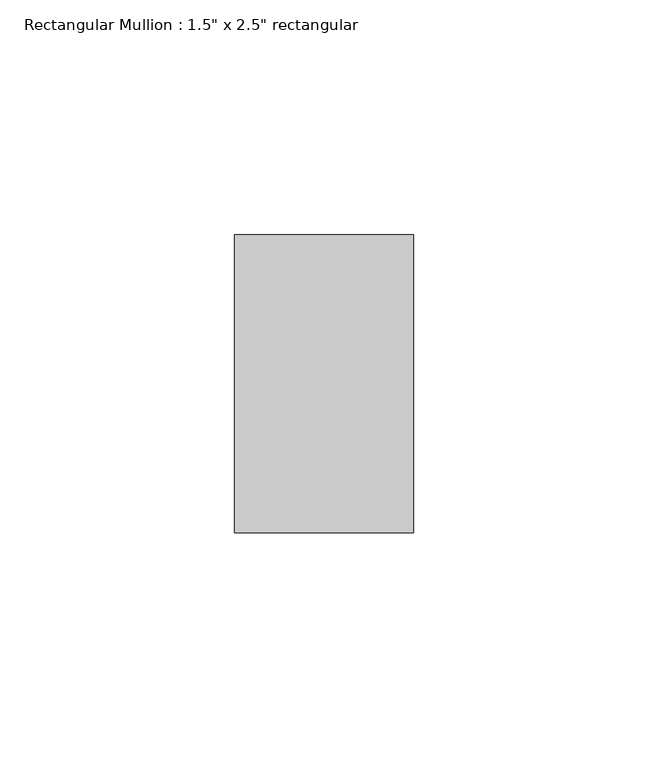
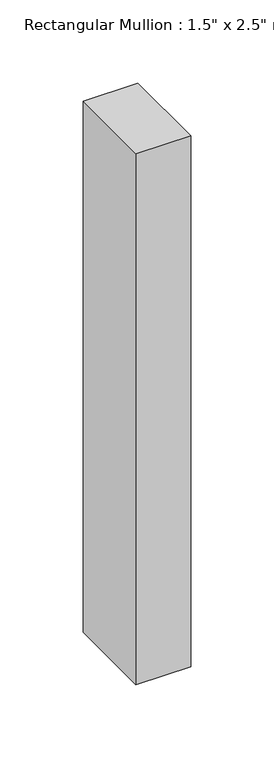
"""IFC4 building model written with IfcOpenShell, lengths in millimetres: member geometry."""

from ifc_helpers import new_model, si_unit, frame, origin, place, context, project, spatial, polyline, outline, extrude, source, transform, mapped, element, save


def member_9157fb7c(model_context):
    return source(origin(), model_context, "Body", "SweptSolid", [
        extrude(outline(polyline([(0.0, 31.75), (0.0, -31.75), (-38.1, -31.75), (-38.1, 31.75), (0.0, 31.75)])), frame((0.0, 0.0, -390.2815409), z_axis=(0.0, 0.0, 1.0), x_axis=(1.0, 0.0, 0.0)), (0.0, 0.0, 1.0), 390.2815409),
    ])


if __name__ == "__main__":
    model = new_model("IFC4")
    model_context = context("Model", 3, world=origin())
    ifc_project = project(units=[si_unit("LENGTHUNIT", "METRE", prefix="MILLI")], contexts=[model_context])
    site = spatial("IfcSite", under=ifc_project)
    building = spatial("IfcBuilding", under=site)
    placement = place(None, origin())
    member_shape = member_9157fb7c(model_context)
    element("IfcMember", 1, ObjectType="Rectangular Mullion : 1.5\" x 2.5\" rectangular", at=placement, inside=building, context=model_context, shape_type="MappedRepresentation", body=[
        mapped(member_shape, transform((0.0, 0.0, 0.0), x_axis=(1.0, 0.0, 0.0), y_axis=(0.0, 1.0, 0.0), z_axis=(0.0, 0.0, 1.0))),
    ])
    save(model, "model.ifc")

# Revit data of these elements
# Type "Rectangular Mullion : 1.5\" x 2.5\" rectangular"
#   built-in parameter 1007304 = 0.208333 (stored number, unit not read)
#   built-in parameter 1007301 = 0.0625 (stored number, unit not read)
#   built-in parameter 1007300 = 0.0625 (stored number, unit not read)
# Element 1 (IfcMember, "Rectangular Mullion : 1.5\" x 2.5\" rectangular")
#   Materials on its faces: "Leather - Black"
# Materials
#   "Leather - Black": class "Generic", colour RGB 40 40 40, transparency 0, Cost = 0
